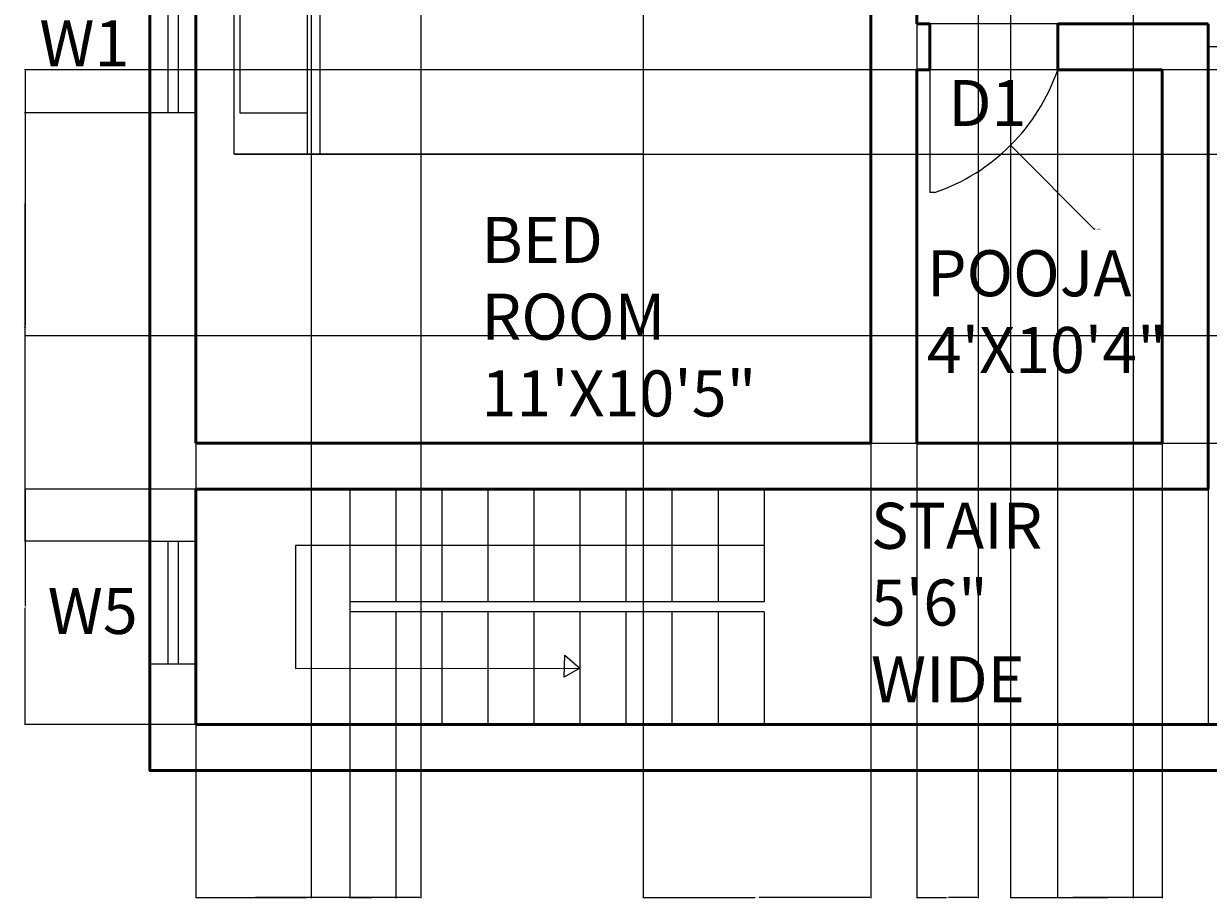
# Model space of a CAD drawing. Units: inches. Extents: x -3 to 419, y -430 to 101.
# Tile 1 of 5: x -3 to 229, y -430 to -259. Entities that reach past the tile are written whole.
import ezdxf

# ---------------------------------------------------------------- set-up
doc = ezdxf.new("R2010")
doc.units = ezdxf.units.IN
doc.header["$MEASUREMENT"] = 0
for name, color, linetype, lineweight in [('A-ANNO-DIMS', 2, 'Continuous', 18), ('A-ANNO-TEXT', 7, 'Continuous', 18), ('A-AREA-IDEN', 7, 'Continuous', 25), ('A-DOOR', 3, 'Continuous', 25), ('A-FLOR-STRS', 7, 'Continuous', 25), ('A-FURN', 8, 'Continuous', 18), ('A-GLAZ', 4, 'Continuous', 25), ('A-WALL', 7, 'Continuous', 50)]:
    doc.layers.add(name, color=color, linetype=linetype, lineweight=lineweight)
doc.styles.get("Standard").update_dxf_attribs({"font": 'arial.ttf'})
doc.dimstyles.get("Standard").update_dxf_attribs({"dimtxt": 0.18, "dimasz": 0.18, "dimexe": 0.18, "dimexo": 0.0625, "dimgap": 0.09, "dimtad": 0, "dimtih": 1, "dimtoh": 1, "dimdec": 4, "dimzin": 0, "dimdsep": 46, "dimtxsty": 'Standard', "dimcen": 0.09, "dimadec": 0, "dimazin": 0, "dimtfac": 1, "dimtdec": 4, "dimtofl": 0, "dimtmove": 0, "dimatfit": 3, "dimfxl": 1, "dimtolj": 1, "dimtzin": 0, "dimarcsym": 0})

# ---------------------------------------------------------------- blocks, each defined once
blk = doc.blocks.new('Bed - Queen')
for p, q in [((0, -80.00003), (0, 0)), ((0, 0), (59.99999, 0)), ((59.99999, 0), (59.99999, -80.00003)), ((7.99999, -1.2), (28.79998, -1.2)), ((7.99999, -14.4), (7.99999, -1.2)), ((28.79998, -1.2), (28.79998, -14.4)), ((31.19999, -1.2), (51.99999, -1.2)), ((31.19999, -14.4), (31.19999, -1.2)), ((51.99999, -1.2), (51.99999, -16.4)), ((0, -14.4), (44.8, -14.4)), ((59.99999, -29.6), (44.8, -14.4)), ((44.8, -14.4), (44.8, -29.6)), ((44.8, -16.8), (0, -16.8)), ((51.99999, -16.4), (46.79936, -16.4)), ((44.8, -29.6), (59.99999, -29.6)), ((59.99999, -80.00003), (0, -80.00003))]:
    blk.add_line(p, q)
blk = doc.blocks.new('WINDOW-24IN')
for p, q in [((0, 5.5), (24, 5.5)), ((0, 3.5), (24, 3.5))]:
    blk.add_line(p, q)
blk.add_lwpolyline([(0, 9), (24, 9), (24, 0), (0, 0)], close=True)
blk = doc.blocks.new('*D26')
at = {"layer": 'A-ANNO-DIMS', "color": 0, "lineweight": -2, "transparency": 16777216}
for p, q in [((171.55, 12.25), (171.55, -429.67)), ((183.55, 12.25), (183.55, -429.67)), ((171.73, -429.49), (177.34, -429.49)), ((183.37, -429.49), (177.76, -429.49))]:
    blk.add_line(p, q, dxfattribs=at)
at = {"layer": 'A-ANNO-DIMS', "color": 0, "transparency": 16777216}
for points in [[(171.73, -429.46), (171.73, -429.52), (171.55, -429.49)], [(183.37, -429.46), (183.37, -429.52), (183.55, -429.49)]]:
    blk.add_solid(points, dxfattribs=at)
at = {"layer": 'Defpoints', "color": 0, "transparency": 16777216}
for p in [(171.55, 12.31), (183.55, 12.31), (183.55, -429.49)]:
    blk.add_point(p, dxfattribs=at)
at = {"layer": 'A-ANNO-DIMS', "color": 0, "transparency": 16777216, "insert": (177.55, -429.49), "char_height": 0.18, "attachment_point": 5}
blk.add_mtext('\\A1;12', dxfattribs=at)
blk = doc.blocks.new('*D30')
at = {"layer": 'A-ANNO-DIMS', "color": 0, "lineweight": -2, "transparency": 16777216}
for p, q in [((21.49, -276.13), (-3, -276.13)), ((-2.82, -276.31), (-2.82, -317.82)), ((-2.82, -359.7), (-2.82, -318.19)), ((21.49, -359.88), (-3, -359.88))]:
    blk.add_line(p, q, dxfattribs=at)
at = {"layer": 'A-ANNO-DIMS', "color": 0, "transparency": 16777216}
for points in [[(-2.85, -276.31), (-2.79, -276.31), (-2.82, -276.13)], [(-2.85, -359.7), (-2.79, -359.7), (-2.82, -359.88)]]:
    blk.add_solid(points, dxfattribs=at)
at = {"layer": 'Defpoints', "color": 0, "transparency": 16777216}
for p in [(21.55, -276.13), (-2.82, -359.88), (21.55, -359.88)]:
    blk.add_point(p, dxfattribs=at)
at = {"layer": 'A-ANNO-DIMS', "color": 0, "transparency": 16777216, "insert": (-2.82, -318), "char_height": 0.18, "attachment_point": 5}
blk.add_mtext('\\A1;83.75', dxfattribs=at)
blk = doc.blocks.new('*D37')
at = {"layer": 'A-ANNO-DIMS', "color": 0, "lineweight": -2, "transparency": 16777216}
for p, q in [((189.86, -65.75), (189.86, -429.67)), ((213.86, -65.75), (213.86, -429.67)), ((190.04, -429.49), (201.64, -429.49)), ((213.68, -429.49), (202.08, -429.49))]:
    blk.add_line(p, q, dxfattribs=at)
at = {"layer": 'A-ANNO-DIMS', "color": 0, "transparency": 16777216}
for points in [[(190.04, -429.46), (190.04, -429.52), (189.86, -429.49)], [(213.68, -429.46), (213.68, -429.52), (213.86, -429.49)]]:
    blk.add_solid(points, dxfattribs=at)
at = {"layer": 'Defpoints', "color": 0, "transparency": 16777216}
for p in [(189.86, -65.69), (213.86, -65.69), (213.86, -429.49)]:
    blk.add_point(p, dxfattribs=at)
at = {"layer": 'A-ANNO-DIMS', "color": 0, "transparency": 16777216, "insert": (201.86, -429.49), "char_height": 0.18, "attachment_point": 5}
blk.add_mtext('\\A1;24', dxfattribs=at)
blk = doc.blocks.new('*D42')
at = {"layer": 'A-ANNO-DIMS', "color": 0, "lineweight": -2, "transparency": 16777216}
for p, q in [((30.49, -349.69), (-3, -349.69)), ((-2.82, -349.87), (-2.82, -372.5)), ((-2.82, -395.51), (-2.82, -372.87)), ((30.49, -395.69), (-3, -395.69))]:
    blk.add_line(p, q, dxfattribs=at)
at = {"layer": 'A-ANNO-DIMS', "color": 0, "transparency": 16777216}
for points in [[(-2.85, -349.87), (-2.79, -349.87), (-2.82, -349.69)], [(-2.85, -395.51), (-2.79, -395.51), (-2.82, -395.69)]]:
    blk.add_solid(points, dxfattribs=at)
at = {"layer": 'Defpoints', "color": 0, "transparency": 16777216}
for p in [(30.55, -349.69), (-2.82, -395.69), (30.55, -395.69)]:
    blk.add_point(p, dxfattribs=at)
at = {"layer": 'A-ANNO-DIMS', "color": 0, "transparency": 16777216, "insert": (-2.82, -372.69), "char_height": 0.18, "attachment_point": 5}
blk.add_mtext('\\A1;46', dxfattribs=at)
blk = doc.blocks.new('*D43')
at = {"layer": 'A-ANNO-DIMS', "color": 0, "lineweight": -2, "transparency": 16777216}
for p, q in [((60.66, -395.75), (60.66, -429.67)), ((69.66, -395.75), (69.66, -429.67)), ((60.84, -429.49), (65.01, -429.49)), ((69.48, -429.49), (65.31, -429.49))]:
    blk.add_line(p, q, dxfattribs=at)
at = {"layer": 'A-ANNO-DIMS', "color": 0, "transparency": 16777216}
for points in [[(60.84, -429.46), (60.84, -429.52), (60.66, -429.49)], [(69.48, -429.46), (69.48, -429.52), (69.66, -429.49)]]:
    blk.add_solid(points, dxfattribs=at)
at = {"layer": 'Defpoints', "color": 0, "transparency": 16777216}
for p in [(60.66, -395.69), (69.66, -395.69), (69.66, -429.49)]:
    blk.add_point(p, dxfattribs=at)
at = {"layer": 'A-ANNO-DIMS', "color": 0, "transparency": 16777216, "insert": (65.16, -429.49), "char_height": 0.18, "attachment_point": 5}
blk.add_mtext('\\A1;9', dxfattribs=at)
blk = doc.blocks.new('*D44')
at = {"layer": 'A-ANNO-DIMS', "color": 0, "lineweight": -2, "transparency": 16777216}
for p, q in [((30.55, -395.75), (30.55, -429.67)), ((60.66, -395.75), (60.66, -429.67)), ((30.73, -429.49), (45.23, -429.49)), ((60.48, -429.49), (45.98, -429.49))]:
    blk.add_line(p, q, dxfattribs=at)
at = {"layer": 'A-ANNO-DIMS', "color": 0, "transparency": 16777216}
for points in [[(30.73, -429.46), (30.73, -429.52), (30.55, -429.49)], [(60.48, -429.46), (60.48, -429.52), (60.66, -429.49)]]:
    blk.add_solid(points, dxfattribs=at)
at = {"layer": 'Defpoints', "color": 0, "transparency": 16777216}
for p in [(30.55, -395.69), (60.66, -395.69), (60.66, -429.49)]:
    blk.add_point(p, dxfattribs=at)
at = {"layer": 'A-ANNO-DIMS', "color": 0, "transparency": 16777216, "insert": (45.61, -429.49), "char_height": 0.18, "attachment_point": 5}
blk.add_mtext('\\A1;30.11', dxfattribs=at)
blk = doc.blocks.new('*D45')
at = {"layer": 'A-ANNO-DIMS', "color": 0, "lineweight": -2, "transparency": 16777216}
for p, q in [((336.49, -267.69), (-3, -267.69)), ((-2.82, -267.87), (-2.82, -293.5)), ((-2.82, -319.5), (-2.82, -293.86)), ((336.49, -319.68), (-3, -319.68))]:
    blk.add_line(p, q, dxfattribs=at)
at = {"layer": 'A-ANNO-DIMS', "color": 0, "transparency": 16777216}
for points in [[(-2.85, -267.87), (-2.79, -267.87), (-2.82, -267.69)], [(-2.85, -319.5), (-2.79, -319.5), (-2.82, -319.68)]]:
    blk.add_solid(points, dxfattribs=at)
at = {"layer": 'Defpoints', "color": 0, "transparency": 16777216}
for p in [(336.55, -267.69), (-2.82, -319.68), (336.55, -319.68)]:
    blk.add_point(p, dxfattribs=at)
at = {"layer": 'A-ANNO-DIMS', "color": 0, "transparency": 16777216, "insert": (-2.82, -293.68), "char_height": 0.18, "attachment_point": 5}
blk.add_mtext('\\A1;51.99', dxfattribs=at)
blk = doc.blocks.new('*D46')
at = {"layer": 'A-ANNO-DIMS', "color": 0, "lineweight": -2, "transparency": 16777216}
for p, q in [((199.09, -267.75), (199.09, -429.67)), ((219.55, -267.75), (219.55, -429.67)), ((199.27, -429.49), (208.93, -429.49)), ((219.37, -429.49), (209.72, -429.49))]:
    blk.add_line(p, q, dxfattribs=at)
at = {"layer": 'A-ANNO-DIMS', "color": 0, "transparency": 16777216}
for points in [[(199.27, -429.46), (199.27, -429.52), (199.09, -429.49)], [(219.37, -429.46), (219.37, -429.52), (219.55, -429.49)]]:
    blk.add_solid(points, dxfattribs=at)
at = {"layer": 'Defpoints', "color": 0, "transparency": 16777216}
for p in [(199.09, -267.69), (219.55, -267.69), (219.55, -429.49)]:
    blk.add_point(p, dxfattribs=at)
at = {"layer": 'A-ANNO-DIMS', "color": 0, "transparency": 16777216, "insert": (209.32, -429.49), "char_height": 0.18, "attachment_point": 5}
blk.add_mtext('\\A1;20.46', dxfattribs=at)
blk = doc.blocks.new('*D51')
at = {"layer": 'A-ANNO-DIMS', "color": 0, "lineweight": -2, "transparency": 16777216}
for p, q in [((53.12, -151.91), (53.12, -429.67)), ((30.55, -157.71), (30.55, -429.67)), ((30.73, -429.49), (41.44, -429.49)), ((52.94, -429.49), (42.23, -429.49))]:
    blk.add_line(p, q, dxfattribs=at)
at = {"layer": 'A-ANNO-DIMS', "color": 0, "transparency": 16777216}
for points in [[(30.73, -429.46), (30.73, -429.52), (30.55, -429.49)], [(52.94, -429.46), (52.94, -429.52), (53.12, -429.49)]]:
    blk.add_solid(points, dxfattribs=at)
at = {"layer": 'Defpoints', "color": 0, "transparency": 16777216}
for p in [(53.12, -151.85), (30.55, -157.64), (30.55, -429.49)]:
    blk.add_point(p, dxfattribs=at)
at = {"layer": 'A-ANNO-DIMS', "color": 0, "transparency": 16777216, "insert": (41.84, -429.49), "char_height": 0.18, "attachment_point": 5}
blk.add_mtext('\\A1;22.57', dxfattribs=at)
blk = doc.blocks.new('*D59')
at = {"layer": 'A-ANNO-DIMS', "color": 0, "lineweight": -2, "transparency": 16777216}
for p, q in [((30.55, 12.25), (30.55, -429.67)), ((74.54, 7.17), (74.54, -429.67)), ((30.73, -429.49), (52.15, -429.49)), ((74.36, -429.49), (52.95, -429.49))]:
    blk.add_line(p, q, dxfattribs=at)
at = {"layer": 'A-ANNO-DIMS', "color": 0, "transparency": 16777216}
for points in [[(30.73, -429.46), (30.73, -429.52), (30.55, -429.49)], [(74.36, -429.46), (74.36, -429.52), (74.54, -429.49)]]:
    blk.add_solid(points, dxfattribs=at)
at = {"layer": 'Defpoints', "color": 0, "transparency": 16777216}
for p in [(30.55, 12.31), (74.54, 7.23), (74.54, -429.49)]:
    blk.add_point(p, dxfattribs=at)
at = {"layer": 'A-ANNO-DIMS', "color": 0, "transparency": 16777216, "insert": (52.55, -429.49), "char_height": 0.18, "attachment_point": 5}
blk.add_mtext('\\A1;43.99', dxfattribs=at)
blk = doc.blocks.new('*D60')
at = {"layer": 'A-ANNO-DIMS', "color": 0, "lineweight": -2, "transparency": 16777216}
for p, q in [((162.55, -245.55), (162.55, -429.67)), ((118.01, -284.25), (118.01, -429.67)), ((118.19, -429.49), (139.88, -429.49)), ((162.37, -429.49), (140.68, -429.49))]:
    blk.add_line(p, q, dxfattribs=at)
at = {"layer": 'A-ANNO-DIMS', "color": 0, "transparency": 16777216}
for points in [[(118.19, -429.46), (118.19, -429.52), (118.01, -429.49)], [(162.37, -429.46), (162.37, -429.52), (162.55, -429.49)]]:
    blk.add_solid(points, dxfattribs=at)
at = {"layer": 'Defpoints', "color": 0, "transparency": 16777216}
for p in [(162.55, -245.49), (118.01, -284.19), (162.55, -429.49)]:
    blk.add_point(p, dxfattribs=at)
at = {"layer": 'A-ANNO-DIMS', "color": 0, "transparency": 16777216, "insert": (140.28, -429.49), "char_height": 0.18, "attachment_point": 5}
blk.add_mtext('\\A1;44.55', dxfattribs=at)
blk = doc.blocks.new('*D64')
at = {"layer": 'A-ANNO-DIMS', "color": 0, "lineweight": -2, "transparency": 16777216}
for p, q in [((38.07, -284.19), (419.21, -284.19)), ((419.03, -284.37), (419.03, -312.25)), ((419.03, -340.51), (419.03, -312.62)), ((30.62, -340.69), (419.21, -340.69))]:
    blk.add_line(p, q, dxfattribs=at)
at = {"layer": 'A-ANNO-DIMS', "color": 0, "transparency": 16777216}
for points in [[(419, -284.37), (419.06, -284.37), (419.03, -284.19)], [(419, -340.51), (419.06, -340.51), (419.03, -340.69)]]:
    blk.add_solid(points, dxfattribs=at)
at = {"layer": 'Defpoints', "color": 0, "transparency": 16777216}
for p in [(38.01, -284.19), (419.03, -284.19), (30.55, -340.69)]:
    blk.add_point(p, dxfattribs=at)
at = {"layer": 'A-ANNO-DIMS', "color": 0, "transparency": 16777216, "insert": (419.03, -312.44), "char_height": 0.18, "attachment_point": 5}
blk.add_mtext('\\A1;56.5', dxfattribs=at)
blk = doc.blocks.new('*D67')
at = {"layer": 'A-ANNO-DIMS', "color": 0, "lineweight": -2, "transparency": 16777216}
for p, q in [((162.46, -255.14), (162.64, -255.14)), ((162.55, -255.23), (162.55, -255.05)), ((206.26, -298.85), (190, -282.59)), ((206.44, -298.85), (206.26, -298.85))]:
    blk.add_line(p, q, dxfattribs=at)
at = {"layer": 'A-ANNO-DIMS', "color": 0, "transparency": 16777216}
blk.add_solid([(190.02, -282.57), (189.97, -282.61), (189.87, -282.46)], dxfattribs=at)
at = {"layer": 'Defpoints', "color": 0, "transparency": 16777216}
for p in [(162.55, -255.14), (189.87, -282.46)]:
    blk.add_point(p, dxfattribs=at)
at = {"layer": 'A-ANNO-DIMS', "color": 0, "transparency": 16777216, "insert": (206.99, -298.85), "char_height": 0.18, "attachment_point": 5}
blk.add_mtext('\\A1;R38.636', dxfattribs=at)

msp = doc.modelspace()

# ---------------------------------------------------------------- linework, layer by layer
at = {"layer": 'A-DOOR'}
for p, q in [((199.0916, -258.6853), (171.5532, -258.6853)), ((269.2198, -263.1853), (228.5532, -263.1853)), ((174.0916, -267.6853), (174.0916, -291.6853)), ((175.0916, -291.6853), (174.0916, -291.6853))]:
    msp.add_line(p, q, dxfattribs=at)
msp.add_arc((162.5485, -255.1422), 38.6359, 288.944375, 341.055625, dxfattribs=at)
at = {"layer": 'A-FLOR-STRS'}
for p, q in [((60.6608, -349.6853), (60.6608, -371.6853)), ((69.6608, -349.6853), (69.6608, -371.6853)), ((78.6608, -349.6853), (78.6608, -371.6853)), ((87.6608, -349.6853), (87.6608, -371.6853)), ((96.6608, -349.6853), (96.6608, -371.6853)), ((105.6608, -349.6853), (105.6608, -371.6853)), ((114.6608, -349.6853), (114.6608, -371.6853)), ((123.6608, -349.6853), (123.6608, -371.6853)), ((132.6608, -349.6853), (132.6608, -371.6853)), ((141.6608, -349.6853), (141.6608, -371.6853)), ((228.5532, -349.6853), (228.5532, -395.6853)), ((141.6608, -360.6853), (50.055, -360.6853)), ((50.055, -360.6853), (50.055, -384.7298)), ((141.6608, -371.6853), (60.6608, -371.6853)), ((60.6608, -371.6853), (60.6608, -373.6853)), ((141.6608, -373.6853), (60.6608, -373.6853)), ((60.6608, -373.6853), (60.6608, -395.6853)), ((69.6608, -373.6853), (69.6608, -395.6853)), ((78.6608, -373.6853), (78.6608, -395.6853)), ((87.6608, -373.6853), (87.6608, -395.6853)), ((96.6608, -373.6853), (96.6608, -395.6853)), ((105.6608, -373.6853), (105.6608, -395.6853)), ((114.6608, -373.6853), (114.6608, -395.6853)), ((123.6608, -373.6853), (123.6608, -395.6853)), ((132.6608, -373.6853), (132.6608, -395.6853)), ((141.6608, -373.6853), (141.6608, -395.6853)), ((102.5904, -386.458), (102.6777, -382.1622)), ((102.6777, -382.1622), (105.6608, -384.6853)), ((50.055, -384.7298), (105.6608, -384.6853)), ((105.6608, -384.6853), (102.5904, -386.458))]:
    msp.add_line(p, q, dxfattribs=at)
at = {"layer": 'A-WALL'}
for p, q in [((171.5532, -258.6853), (171.5532, -192.6713)), ((30.5532, -286.6853), (30.5532, -215.6853)), ((162.5532, -267.6853), (162.5532, -245.4865)), ((174.0916, -258.6853), (171.5532, -258.6853)), ((174.0916, -267.6853), (174.0916, -258.6853)), ((219.5532, -258.6853), (199.0916, -258.6853)), ((199.0916, -267.6853), (199.0916, -258.6853)), ((228.5532, -258.6853), (219.5532, -258.6853)), ((228.5532, -267.6853), (228.5532, -258.6853)), ((162.5532, -267.6853), (162.5532, -286.6853)), ((171.5532, -267.6853), (171.5532, -286.6853)), ((174.0916, -267.6853), (171.5532, -267.6853)), ((219.5532, -267.6853), (199.0916, -267.6853)), ((219.5532, -286.6853), (219.5532, -267.6853)), ((228.5532, -267.6853), (228.5532, -340.6853)), ((30.5532, -286.6853), (30.5532, -295.6853)), ((162.5532, -286.6853), (162.5532, -340.6853)), ((171.5532, -286.6853), (171.5532, -340.6853)), ((219.5532, -286.6853), (219.5532, -340.6853)), ((30.5532, -340.6853), (30.5532, -295.6853)), ((30.5532, -340.6853), (162.5532, -340.6853)), ((171.5532, -340.6853), (219.5532, -340.6853)), ((228.5532, -349.6853), (228.5532, -340.6853)), ((30.5532, -395.6853), (30.5532, -349.6853)), ((30.5532, -349.6853), (162.5532, -349.6853)), ((162.5532, -349.6853), (228.5532, -349.6853)), ((267.5221, -395.6853), (30.5532, -395.6853))]:
    msp.add_line(p, q, dxfattribs=at)
msp.add_lwpolyline([(266.5221, -404.6853), (21.5532, -404.6853), (21.5532, 21.3147), (345.5532, 21.3147), (345.5532, -404.6853)], dxfattribs=at)

# ---------------------------------------------------------------- block references
at = {"layer": 'A-FURN', "rotation": 90}
msp.add_blockref('Bed - Queen', (38.0056, -284.1853), dxfattribs=at)
at = {"layer": 'A-GLAZ'}
for p, rotation in [((21.5535, -252.131), 269.9999999999999), ((21.5535, -359.8767), 270.0000000000001)]:
    msp.add_blockref('WINDOW-24IN', p, dxfattribs=dict(at, rotation=rotation))

# ---------------------------------------------------------------- texts
at = {"layer": 'A-ANNO-TEXT', "char_height": 9, "attachment_point": 1}
for s, width, insert in [('W1', 37.451717, (-0.0716, -258.0081)), ('D1', 11.357564, (177.7135, -269.6912)), ('W5', 14.772715, (1.5675, -368.9932))]:
    msp.add_mtext_dynamic_manual_height_columns(s, width=width, gutter_width=45, heights=[0], dxfattribs=dict(at, insert=insert))
at = {"layer": 'A-AREA-IDEN', "char_height": 9, "attachment_point": 1}
for s, width, insert in [('BED ROOM\\P11\'X10\'5"', 53.114163, (86.402, -296.4549)), ('POOJA\\P4\'X10\'4"', 33.025411, (173.5063, -302.9692)), ('STAIR\\P5\'6" WIDE', 35.865585, (162.5778, -352.3436))]:
    msp.add_mtext_dynamic_manual_height_columns(s, width=width, gutter_width=45, heights=[0], dxfattribs=dict(at, insert=insert))

# ---------------------------------------------------------------- dimensions: what is measured, and where the dimension line sits
at = {"layer": 'A-ANNO-DIMS'}
for base, p1, p2, override, picture, middle in [((74.5439, -429.4854), (30.5532, 12.3147), (74.5439, 7.23), {"dimdec": 2, "dimlfac": 1, "dimrnd": 0, "dimzin": 0, "dimdsep": 46, "dimlunit": 2}, '*D59', (52.5485, -429.4854)), ((183.5532, -429.4854), (171.5532, 12.3147), (183.5532, 12.3147), {"dimdec": 0, "dimlfac": 1, "dimrnd": 0, "dimzin": 0, "dimdsep": 46, "dimlunit": 2}, '*D26', (177.5532, -429.4854)), ((213.8603, -429.4854), (189.8603, -65.6853), (213.8603, -65.6853), {"dimdec": 0, "dimlfac": 1, "dimrnd": 0, "dimzin": 0, "dimdsep": 46, "dimlunit": 2}, '*D37', (201.8603, -429.4854)), ((30.5532, -429.4854), (53.124, -151.8457), (30.5532, -157.6432), {"dimdec": 2, "dimlfac": 1, "dimrnd": 0, "dimzin": 0, "dimdsep": 46, "dimlunit": 2}, '*D51', (41.8386, -429.4854)), ((162.5532, -429.4854), (118.0057, -284.1853), (162.5532, -245.4865), {"dimdec": 2, "dimlfac": 1, "dimrnd": 0, "dimzin": 0, "dimdsep": 46, "dimlunit": 2}, '*D60', (140.2794, -429.4854)), ((219.5532, -429.4854), (199.0916, -267.6853), (219.5532, -267.6853), {"dimdec": 2, "dimlfac": 1, "dimrnd": 0, "dimzin": 0, "dimdsep": 46, "dimlunit": 2}, '*D46', (209.3224, -429.4854)), ((60.6608, -429.4854), (30.5532, -395.6853), (60.6608, -395.6853), {"dimdec": 2, "dimlfac": 1, "dimrnd": 0, "dimzin": 0, "dimdsep": 46, "dimlunit": 2}, '*D44', (45.607, -429.4854)), ((69.6608, -429.4854), (60.6608, -395.6853), (69.6608, -395.6853), {"dimdec": 0, "dimlfac": 1, "dimrnd": 0, "dimzin": 0, "dimdsep": 46, "dimlunit": 2}, '*D43', (65.1608, -429.4854))]:
    dim = msp.add_linear_dim(base=base, p1=p1, p2=p2, dimstyle='Standard', override=override, dxfattribs=at)
    dim.commit()
    dim.dimension.update_dxf_attribs({"geometry": picture, "text_midpoint": middle})
dim = msp.add_radius_dim(center=(162.5485, -255.1422), mpoint=(189.868, -282.462), dimstyle='Standard', override={"dimdec": 3, "dimlfac": 1, "dimrnd": 0, "dimzin": 0, "dimdsep": 46, "dimlunit": 2}, dxfattribs=at)
dim.commit()
dim.dimension.update_dxf_attribs({"geometry": '*D67', "text_midpoint": (206.9894, -298.8539), "dimtype": 164})
for base, p1, p2, override, picture, middle in [((-2.8238, -319.6772), (336.5532, -267.6853), (336.5532, -319.6772), {"dimdec": 2, "dimlfac": 1, "dimrnd": 0, "dimzin": 0, "dimdsep": 46, "dimlunit": 2}, '*D45', (-2.8238, -293.6812)), ((-2.8238, -359.8765), (21.5532, -276.1309), (21.5532, -359.8765), {"dimdec": 2, "dimlfac": 1, "dimrnd": 0, "dimzin": 0, "dimdsep": 46, "dimlunit": 2}, '*D30', (-2.8238, -318.0037)), ((419.0271, -284.1853), (30.5532, -340.6853), (38.0056, -284.1853), {"dimdec": 1, "dimlfac": 1, "dimrnd": 0, "dimzin": 0, "dimdsep": 46, "dimlunit": 2}, '*D64', (419.0271, -312.4353)), ((-2.8238, -395.6853), (30.5532, -349.6853), (30.5532, -395.6853), {"dimdec": 0, "dimlfac": 1, "dimrnd": 0, "dimzin": 0, "dimdsep": 46, "dimlunit": 2}, '*D42', (-2.8238, -372.6853))]:
    dim = msp.add_linear_dim(base=base, p1=p1, p2=p2, angle=90, dimstyle='Standard', override=override, dxfattribs=at)
    dim.commit()
    dim.dimension.update_dxf_attribs({"geometry": picture, "text_midpoint": middle})

doc.saveas('drawing.dxf')
